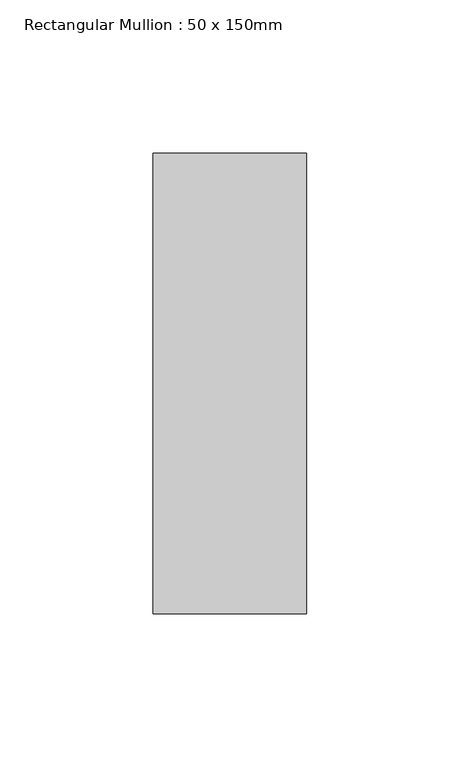
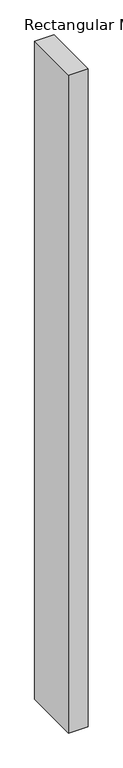
"""IFC4 building model written with IfcOpenShell, lengths in millimetres: member geometry, Rectangular Mullion : 50 x 150mm."""

from ifc_helpers import new_model, si_unit, frame, origin, place, context, project, spatial, polyline, outline, extrude, source, transform, mapped, element, save


def rectangular_mullion_50_x_150mm_ded00a16(model_context):
    return source(origin(), model_context, "Body", "SweptSolid", [
        extrude(outline(polyline([(0.0, 75.0), (0.0, -75.0), (-50.0, -75.0), (-50.0, 75.0), (0.0, 75.0)])), frame((0.0, 0.0, -1780.0), z_axis=(0.0, 0.0, 1.0), x_axis=(1.0, 0.0, 0.0)), (0.0, 0.0, 1.0), 1780.0),
    ])


if __name__ == "__main__":
    model = new_model("IFC4")
    model_context = context("Model", 3, world=origin())
    ifc_project = project(units=[si_unit("LENGTHUNIT", "METRE", prefix="MILLI")], contexts=[model_context])
    site = spatial("IfcSite", under=ifc_project)
    building = spatial("IfcBuilding", under=site)
    placement = place(None, origin())
    rectangular_mullion_50_x_150mm_shape = rectangular_mullion_50_x_150mm_ded00a16(model_context)
    element("IfcMember", 1, ObjectType="Rectangular Mullion : 50 x 150mm", at=placement, inside=building, context=model_context, shape_type="MappedRepresentation", body=[
        mapped(rectangular_mullion_50_x_150mm_shape, transform((0.0, 0.0, 0.0), x_axis=(1.0, 0.0, 0.0), y_axis=(0.0, 1.0, 0.0), z_axis=(0.0, 0.0, 1.0))),
    ])
    save(model, "model.ifc")

# Revit data of these elements
# Type "Rectangular Mullion : 50 x 150mm"
#   built-in parameter 1007304 = 0.492126 (stored number, unit not read)
#   built-in parameter 1007301 = 0.082021 (stored number, unit not read)
#   built-in parameter 1007300 = 0.082021 (stored number, unit not read)
# Element 1 (IfcMember, "Rectangular Mullion : 50 x 150mm")
#   Materials on its faces: "Aluminium"
# Materials
#   "Aluminium": class "Metal", colour RGB 247 247 247, transparency 0, Description = "Aluminium 6061", Cost = 0
